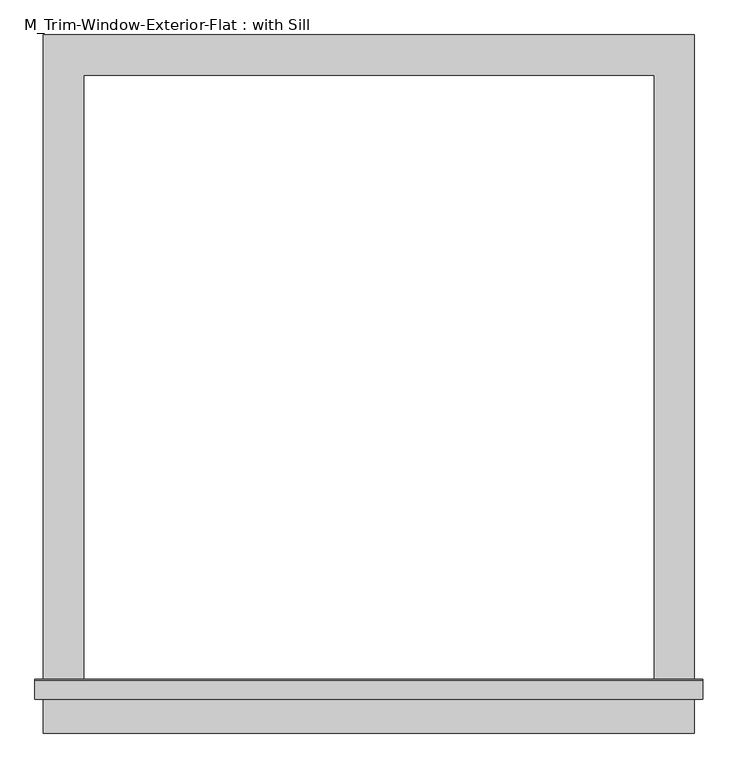
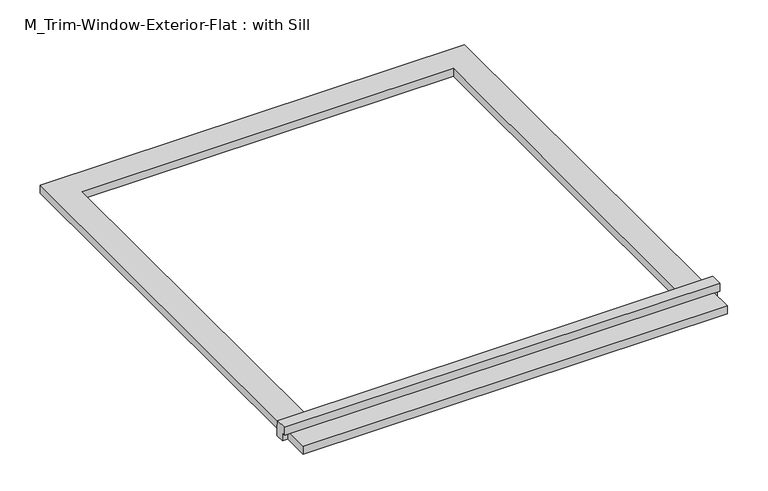
"""IFC4 building model written with IfcOpenShell, lengths in millimetres: proxy geometry, M_Trim-Window-Exterior-Flat : with Sill."""

from ifc_helpers import new_model, si_unit, frame, origin, origin_with_axes, place, context, project, spatial, polyline, outline, extrude, source, transform, mapped, element, save


def m_trim_window_exterior_flat_with_sill_90d3a428(model_context):
    return source(origin(), model_context, "Body", "SweptSolid", [
        extrude(outline(polyline([(485.0, -920.4323709), (485.0, -980.4323709), (-485.0, -980.4323709), (-485.0, -920.4323709), (485.0, -920.4323709)])), origin_with_axes(), (0.0, 0.0, 1.0), 19.05),
        extrude(outline(polyline([(-930.0, 38.1), (-902.4580645, 38.1), (-900.0, 19.05), (-900.0, 0.0), (-920.4323709, 0.0), (-920.4323709, 19.05), (-930.0, 19.05), (-930.0, 38.1)])), frame((-497.7, 0.0, 0.0), z_axis=(1.0, 0.0, 0.0), x_axis=(0.0, 1.0, 0.0)), (0.0, 0.0, 1.0), 995.4),
        extrude(outline(polyline([(-485.0, 60.0), (485.0, 60.0), (485.0, -900.0), (425.0, -900.0), (425.0, 0.0), (-425.0, 0.0), (-425.0, -900.0), (-485.0, -900.0), (-485.0, 60.0)])), origin_with_axes(), (0.0, 0.0, 1.0), 19.05),
    ])


if __name__ == "__main__":
    model = new_model("IFC4")
    model_context = context("Model", 3, world=origin())
    ifc_project = project(units=[si_unit("LENGTHUNIT", "METRE", prefix="MILLI")], contexts=[model_context])
    site = spatial("IfcSite", under=ifc_project)
    building = spatial("IfcBuilding", under=site)
    placement = place(None, origin())
    m_trim_window_exterior_flat_with_sill_shape = m_trim_window_exterior_flat_with_sill_90d3a428(model_context)
    element("IfcBuildingElementProxy", 1, Name="M_Trim-Window-Exterior-Flat : with Sill", ObjectType="M_Trim-Window-Exterior-Flat : with Sill", at=placement, inside=building, context=model_context, shape_type="MappedRepresentation", body=[
        mapped(m_trim_window_exterior_flat_with_sill_shape, transform((0.0, 0.0, 0.0), x_axis=(1.0, 0.0, 0.0), y_axis=(0.0, 1.0, 0.0), z_axis=(0.0, 0.0, 1.0))),
    ])
    save(model, "model.ifc")

# Revit data of these elements
# Type "M_Trim-Window-Exterior-Flat : with Sill"
#   Trim Width = 0.19685 ft
#   Trim Thickness_Picture Frame = 0.098425 ft
#   Trim Thickness_with Sill = 0.0625 ft
#   Sill Thickness = 0.098425 ft
#   Opening Width [instance default] = 1.968504 ft
#   Opening Height [instance default] = 2.952756 ft
#   Default Elevation = 3.937008 ft
#   Sill = yes
#   Picture Frame = no
#   Trim Material [instance default] = none
# Element 1 (IfcBuildingElementProxy, "M_Trim-Window-Exterior-Flat : with Sill")
#   Opening Width = 2.788714 ft
#   Trim Material = Clad - White
#   Materials on its faces: "Clad - White"
# Materials
#   "Clad - White": class "Wood", colour RGB 242 242 238, transparency 0, Cost = 0
